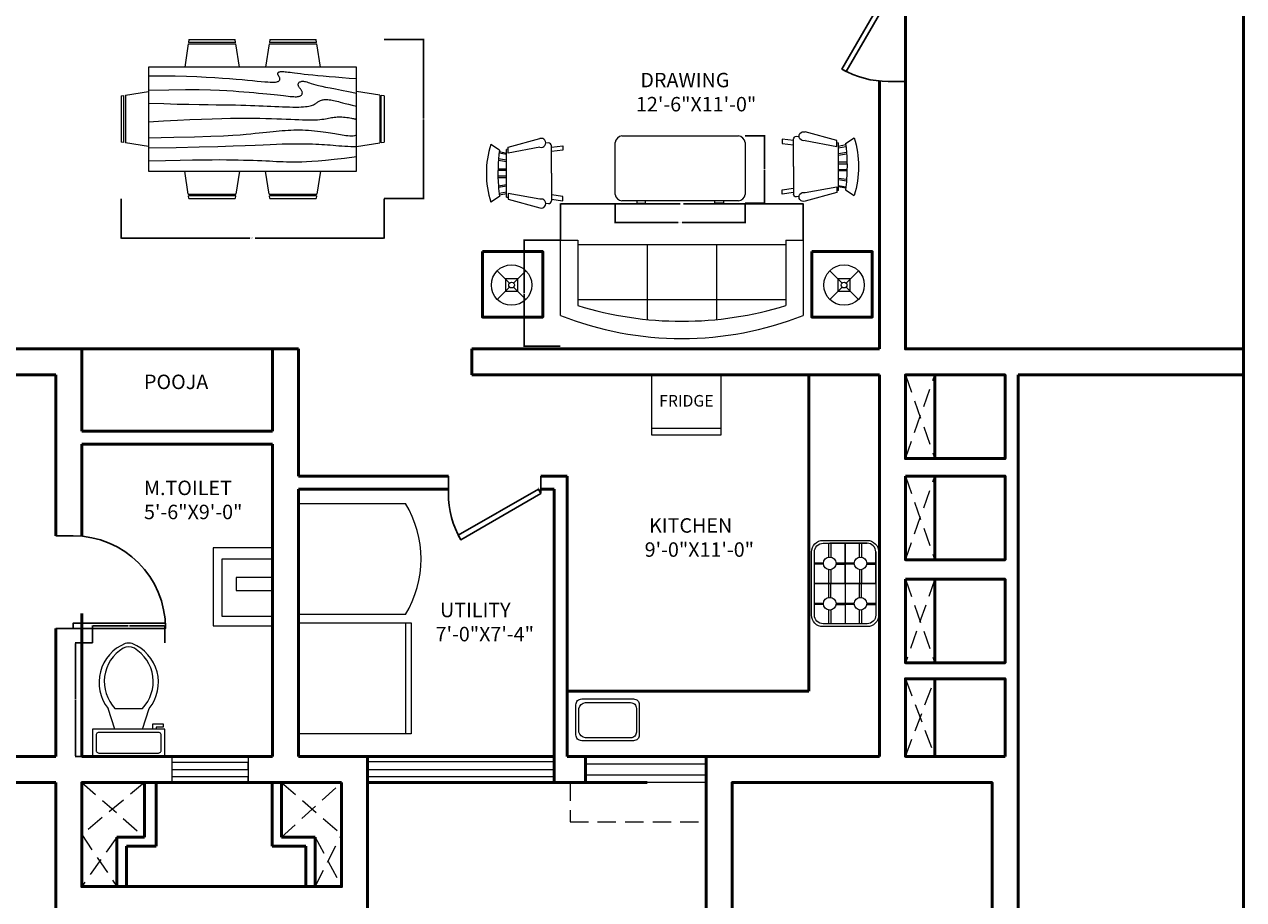
# Model space of a CAD drawing. Units: inches. Extents: x -105 to 1531, y -656 to 2003.
# Tile 4 of 6: x 553 to 975, y 553 to 856. Entities that reach past the tile are written whole.
import ezdxf

# ---------------------------------------------------------------- set-up
doc = ezdxf.new("R2010")
doc.units = ezdxf.units.IN
doc.header["$MEASUREMENT"] = 0
doc.linetypes.add('DASHED', pattern=[19.05, 12.7, -6.35])
for name, color, linetype, lineweight in [('A-ANNO-DIMS', 2, 'Continuous', 18), ('A-AREA-IDEN', 7, 'Continuous', 25), ('A-DOOR', 3, 'Continuous', 25), ('A-FLOR-FIXT', 9, 'Continuous', 18), ('A-FLOR-OVHD', 8, 'DASHED', 18), ('A-FURN', 8, 'Continuous', 18), ('A-GLAZ', 4, 'Continuous', 18), ('A-WALL', 7, 'Continuous', 50)]:
    doc.layers.add(name, color=color, linetype=linetype, lineweight=lineweight)
doc.styles.get("Standard").update_dxf_attribs({"font": 'arial.ttf'})
doc.dimstyles.get("Standard").update_dxf_attribs({"dimtxt": 0.18, "dimasz": 0.18, "dimexe": 0.18, "dimexo": 0.0625, "dimgap": 0.09, "dimtad": 0, "dimtih": 1, "dimtoh": 1, "dimdec": 0, "dimzin": 0, "dimdsep": 46, "dimlunit": 3, "dimtxsty": 'Standard', "dimcen": 0.09, "dimadec": 0, "dimazin": 0, "dimtfac": 1, "dimtdec": 0, "dimtofl": 0, "dimtmove": 0, "dimatfit": 3, "dimfxl": 1, "dimtolj": 1, "dimtzin": 0, "dimarcsym": 0})

# ---------------------------------------------------------------- blocks, each defined once
blk = doc.blocks.new('Dining Set - 36 x 72 in.')
for p, q in [((-22.2343, 26.00059), (-23.4847, 17.99762)), ((-22.2304, 26), (-5.7608, 26)), ((-22, 27.5), (-22.1562, 26.50042)), ((-5.8416, 26.5), (-22.1534, 26.5)), ((-22, 27.5), (-6, 27.5)), ((-5.8437, 26.49966), (-6, 27.5)), ((-4.5152, 17.99762), (-5.7655, 25.99926)), ((5.7657, 26.00059), (4.5153, 17.99762)), ((5.7696, 26), (22.2392, 26)), ((6, 27.5), (5.8438, 26.50042)), ((22.1584, 26.5), (5.8466, 26.5)), ((6, 27.5), (22, 27.5)), ((22.1563, 26.49966), (22, 27.5)), ((23.4848, 17.99762), (22.2345, 25.99926)), ((36, 18), (-36, 18)), ((-36, 18), (-36, -18)), ((36, -18), (36, 18)), ((-44.0006, 8.23428), (-35.9976, 9.48474)), ((44.0006, 8.23428), (35.9976, 9.48474)), ((-45.5, 8), (-44.5004, 8.15617)), ((-45.5, 8), (-45.5, -8)), ((-44.5, -8.15843), (-44.5, 8.15338)), ((-44, 8.23041), (-44, -8.23915)), ((44, 8.23041), (44, -8.23915)), ((44.5, -8.15843), (44.5, 8.15338)), ((45.5, 8), (44.5005, 8.15617)), ((45.5, 8), (45.5, -8)), ((-44.4997, -8.15631), (-45.5, -8)), ((-35.9976, -9.48476), (-43.9993, -8.2345)), ((35.9976, -9.48476), (43.9993, -8.2345)), ((44.4997, -8.15631), (45.5, -8)), ((-36, -18), (36, -18)), ((-22.2343, -26.0006), (-23.4847, -17.99762)), ((-4.5152, -17.99762), (-5.7655, -25.99928)), ((5.7657, -26.0006), (4.5153, -17.99762)), ((23.4848, -17.99762), (22.2345, -25.99928)), ((-22.2304, -26), (-5.7608, -26)), ((-22, -27.5), (-22.1562, -26.50044)), ((-5.8416, -26.5), (-22.1534, -26.5)), ((-22, -27.5), (-6, -27.5)), ((-5.8437, -26.49967), (-6, -27.5)), ((5.7696, -26), (22.2392, -26)), ((6, -27.5), (5.8438, -26.50044)), ((22.1584, -26.5), (5.8466, -26.5)), ((6, -27.5), (22, -27.5)), ((22.1563, -26.49967), (22, -27.5))]:
    blk.add_line(p, q)
for points in [[(-36, 15), (-31.1772, 14.97754), (-26.8079, 14.91406), (-22.8538, 14.81543), (-19.276, 14.6875), (-16.0362, 14.53613), (-13.0957, 14.36718), (-10.4159, 14.18652), (-7.9583, 14), (-5.6904, 13.81315), (-3.6035, 13.63021), (-1.6954, 13.45508), (0.0365, 13.29166), (1.5945, 13.14388), (2.9811, 13.01562), (4.1988, 12.9108), (5.25, 12.83333), (6.1393, 12.78613), (6.8802, 12.76823), (7.4883, 12.77767), (7.9792, 12.8125), (8.3685, 12.87077), (8.6719, 12.95052), (8.9049, 13.0498), (9.0833, 13.16666), (9.2205, 13.29899), (9.3216, 13.44401), (9.3895, 13.59879), (9.4271, 13.76041), (9.4373, 13.92594), (9.4232, 14.09245), (9.3875, 14.257), (9.3333, 14.41666), (9.2638, 14.56917), (9.1836, 14.71484), (9.0975, 14.85465), (9.0104, 14.98958), (8.9272, 15.1206), (8.8529, 15.2487), (8.7922, 15.37483), (8.75, 15.5), (8.7305, 15.62467), (8.7344, 15.74739), (8.7617, 15.86621), (8.8125, 15.97916), (8.8867, 16.08431), (8.9844, 16.17968), (9.1055, 16.26334), (9.25, 16.33333), (9.4189, 16.38802), (9.6172, 16.42708), (9.8506, 16.45052), (10.125, 16.45833), (10.4463, 16.45052), (10.8203, 16.42708), (11.2529, 16.38802), (11.75, 16.33333), (12.3184, 16.26318), (12.9694, 16.17838), (13.7151, 16.07991), (14.5677, 15.96875), (15.5395, 15.84586), (16.6426, 15.71224), (17.8893, 15.56884), (19.2917, 15.41666), (20.859, 15.25667), (22.5879, 15.08984), (24.4721, 14.91715), (26.5052, 14.73958), (28.6809, 14.5581), (30.9929, 14.3737), (33.4347, 14.18733), (36, 14)], [(-36, 10), (-28.9766, 10.14274), (-23.1725, 10.20442), (-18.4241, 10.19775), (-14.5677, 10.13541), (-11.4399, 10.03011), (-8.877, 9.89453), (-6.7154, 9.74137), (-4.7917, 9.58333), (-2.9698, 9.43082), (-1.2246, 9.28515), (0.4415, 9.14534), (2.026, 9.01041), (3.5266, 8.87939), (4.9408, 8.7513), (6.266, 8.62516), (7.5, 8.5), (8.6411, 8.37549), (9.6914, 8.2539), (10.6538, 8.13818), (11.5312, 8.03125), (12.3267, 7.93603), (13.043, 7.85547), (13.6831, 7.79248), (14.25, 7.75), (14.7471, 7.7303), (15.1797, 7.73307), (15.5537, 7.75732), (15.875, 7.80208), (16.1494, 7.86637), (16.3828, 7.94922), (16.5811, 8.04964), (16.75, 8.16666), (16.8944, 8.29915), (17.0143, 8.44531), (17.1089, 8.60319), (17.1771, 8.77083), (17.218, 8.94629), (17.2305, 9.1276), (17.2137, 9.31282), (17.1667, 9.5), (17.0895, 9.6875), (16.987, 9.875), (16.8649, 10.0625), (16.7292, 10.25), (16.5856, 10.4375), (16.4401, 10.625), (16.2985, 10.8125), (16.1667, 11), (16.05, 11.18733), (15.9518, 11.3737), (15.8752, 11.5581), (15.8229, 11.73958), (15.798, 11.91715), (15.8034, 12.08984), (15.842, 12.25667), (15.9167, 12.41666), (16.0295, 12.56836), (16.1784, 12.70833), (16.3605, 12.83268), (16.5729, 12.9375), (16.8127, 13.01888), (17.0768, 13.07291), (17.3625, 13.0957), (17.6667, 13.08333), (17.9894, 13.03312), (18.3418, 12.94726), (18.7382, 12.82918), (19.1927, 12.68229), (19.7195, 12.51001), (20.3327, 12.31575), (21.0465, 12.10294), (21.875, 11.875), (22.8357, 11.63354), (23.959, 11.37304), (25.2786, 11.08618), (26.8282, 10.76562), (28.6414, 10.40405), (30.752, 9.99414), (33.1936, 9.52856), (36, 9)], [(-36, 5.5), (-30.7157, 5.3348), (-26.069, 5.20963), (-21.9946, 5.11767), (-18.4271, 5.05208), (-15.3009, 5.00602), (-12.5508, 4.97265), (-10.1112, 4.94515), (-7.9167, 4.91666), (-5.909, 4.88167), (-4.0586, 4.83984), (-2.3429, 4.79215), (-0.7396, 4.73958), (0.7739, 4.6831), (2.22, 4.6237), (3.6213, 4.56233), (5, 4.5), (6.373, 4.43782), (7.7344, 4.3776), (9.0723, 4.32129), (10.375, 4.27083), (11.6309, 4.22819), (12.8281, 4.19531), (13.9551, 4.17415), (15, 4.16666), (15.954, 4.17448), (16.819, 4.19791), (17.6001, 4.23698), (18.3021, 4.29166), (18.9299, 4.36198), (19.4883, 4.44791), (19.9823, 4.54948), (20.4167, 4.66666), (20.7969, 4.79899), (21.1302, 4.94401), (21.4245, 5.09879), (21.6875, 5.26041), (21.9271, 5.42594), (22.1511, 5.59245), (22.3672, 5.757), (22.5834, 5.91666), (22.8065, 6.06868), (23.0404, 6.21093), (23.2879, 6.34147), (23.5521, 6.45833), (23.8358, 6.55957), (24.142, 6.64323), (24.4735, 6.70735), (24.8334, 6.75), (25.2235, 6.76969), (25.642, 6.76692), (26.0858, 6.74267), (26.5521, 6.69791), (27.0379, 6.63362), (27.5404, 6.55078), (28.0565, 6.45036), (28.5834, 6.33333), (29.1242, 6.19987), (29.7071, 6.04687), (30.3661, 5.87044), (31.1354, 5.66666), (32.0493, 5.43164), (33.142, 5.16146), (34.4475, 4.85221), (36, 4.5)], [(-36, -1), (-30.7915, -0.6591), (-26.0195, -0.38216), (-21.6519, -0.16284), (-17.6563, 0.00521), (-14.0005, 0.12833), (-10.6523, 0.21289), (-7.5796, 0.26522), (-4.75, 0.29166), (-2.134, 0.29793), (0.2878, 0.28711), (2.5317, 0.26163), (4.6146, 0.22396), (6.5529, 0.17651), (8.3633, 0.12174), (10.0623, 0.06209), (11.6667, 0), (13.1899, -0.06201), (14.6341, -0.1211), (15.9982, -0.17432), (17.2813, -0.21875), (18.4823, -0.25147), (19.6003, -0.26953), (20.6343, -0.27002), (21.5834, -0.25), (22.4481, -0.20768), (23.2357, -0.14584), (23.9549, -0.06836), (24.6146, 0.02083), (25.2235, 0.11784), (25.7904, 0.21875), (26.3241, 0.31966), (26.8334, 0.41666), (27.3265, 0.50618), (27.8099, 0.58593), (28.2894, 0.65397), (28.7709, 0.70833), (29.2601, 0.74707), (29.763, 0.76823), (30.2855, 0.76985), (30.8334, 0.75), (31.4088, 0.70784), (31.9994, 0.64713), (32.589, 0.57275), (33.1615, 0.48958), (33.7008, 0.4025), (34.1908, 0.3164), (34.6153, 0.23616), (34.9584, 0.16666), (35.2099, 0.11165), (35.3848, 0.07031), (35.504, 0.04069), (35.5886, 0.02083), (35.6594, 0.00879), (35.7377, 0.0026), (35.8442, 0.00032), (36, 0)], [(-36, -6.5), (-27.1843, -6.31267), (-20.084, -6.1263), (-14.469, -5.9419), (-10.1094, -5.76042), (-6.7752, -5.58285), (-4.2363, -5.41016), (-2.2629, -5.24333), (-0.625, -5.08334), (0.8708, -4.93099), (2.2715, -4.78646), (3.5872, -4.64974), (4.8281, -4.52084), (6.0046, -4.39974), (7.127, -4.28646), (8.2053, -4.18099), (9.25, -4.08334), (10.2705, -3.99382), (11.2734, -3.91407), (12.2647, -3.84603), (13.25, -3.79167), (14.2354, -3.75293), (15.2266, -3.73177), (16.2295, -3.73015), (17.25, -3.75), (18.2912, -3.79248), (19.3451, -3.85547), (20.4009, -3.93604), (21.4479, -4.03125), (22.4754, -4.13819), (23.4727, -4.25391), (24.4289, -4.37549), (25.3334, -4.5), (26.1785, -4.62492), (26.9694, -4.74935), (27.7145, -4.87281), (28.4219, -4.99479), (29.1, -5.11483), (29.7572, -5.23242), (30.4016, -5.34709), (31.0417, -5.45834), (31.6837, -5.56437), (32.3262, -5.65821), (32.9658, -5.73153), (33.599, -5.77604), (34.2224, -5.78345), (34.8327, -5.74545), (35.4264, -5.65373), (36, -5.5)], [(-36, -10), (-26.4022, -9.81299), (-18.4675, -9.62891), (-11.9839, -9.45069), (-6.7396, -9.28125), (-2.5226, -9.12354), (0.8789, -8.98047), (3.6769, -8.85498), (6.0833, -8.75), (8.2767, -8.66765), (10.3021, -8.60677), (12.1712, -8.56543), (13.8958, -8.54167), (15.4876, -8.53353), (16.9583, -8.53907), (18.3197, -8.55632), (19.5834, -8.58334), (20.7616, -8.61841), (21.8685, -8.66081), (22.9188, -8.71004), (23.9271, -8.76563), (24.9081, -8.82707), (25.8763, -8.89388), (26.8465, -8.96558), (27.8334, -9.04167), (28.8474, -9.12118), (29.8828, -9.20117), (30.93, -9.27824), (31.9792, -9.34896), (33.0205, -9.40991), (34.0443, -9.45768), (35.0407, -9.48885), (36, -9.5)], [(-36, -14.5), (-30.0881, -14.33513), (-25.0332, -14.21224), (-20.7312, -14.12647), (-17.0781, -14.07292), (-13.97, -14.04671), (-11.3027, -14.04297), (-8.9724, -14.05681), (-6.875, -14.08334), (-4.9224, -14.11833), (-3.0905, -14.16016), (-1.3709, -14.20785), (0.2448, -14.26042), (1.7647, -14.3169), (3.1973, -14.3763), (4.5507, -14.43767), (5.8333, -14.5), (7.0554, -14.5621), (8.235, -14.62175), (9.3922, -14.67652), (10.5469, -14.72396), (11.7192, -14.76164), (12.929, -14.78711), (14.1965, -14.79794), (15.5417, -14.79167), (16.9933, -14.76424), (18.6152, -14.70508), (20.4804, -14.60197), (22.6615, -14.44271), (25.2312, -14.21509), (28.2624, -13.9069), (31.8277, -13.50594), (36, -13)]]:
    blk.add_lwpolyline(points)
blk = doc.blocks.new('Sofa - Roundback 7 ft.')
for p, q in [((-12.00002, -32.4421), (-12.00003, -6.5971)), ((11.99997, -32.4421), (11.99998, -6.5971)), ((-36.000027, -34), (-36.000027, -11.4696)), ((35.99998, -34), (35.99998, -11.4696)), ((-35.999844, -13.3819), (35.9998, -13.3819)), ((-36.000027, -32.4421), (35.99998, -32.4421))]:
    blk.add_line(p, q)
for points in [[(-36.000027, -34), (-42.000027, -34), (-42.000027, -8)], [(41.99998, -8), (41.99998, -34), (35.99998, -34)]]:
    blk.add_lwpolyline(points)
for centre, radius, start, end in [((0, -114.25), 114.25, 68.43141, 111.5686), ((-0.00001, -127.1968), 121.1968, 72.72033, 107.2797)]:
    blk.add_arc(centre, radius, start, end)
blk = doc.blocks.new('Chair - Rocking')
for p, q in [((-8, -4.5), (-10, -1.5)), ((-4.5, -7), (-4.96674, -4.19951)), ((-4, -7), (-4.40532, -4.16272)), ((-1.5, -4.05012), (-1.5, -7)), ((-1, -7), (-1, -4.05012)), ((1, -7), (1, -4.04655)), ((1.5, -4.05012), (1.5, -7)), ((4, -7), (4.40187, -4.18694)), ((4.5, -7), (4.96761, -4.19437)), ((8, -4.5), (10, -1.5)), ((-9, -7.5), (-12, -18.49999)), ((-7, -7.5), (-9, -7.5)), ((-9, -18.49999), (-7, -7.5)), ((-8.23428, -6.99939), (-8.3093, -7.47958)), ((-8.23041, -7), (8.23915, -7)), ((-7.5, -4.5), (-7, -7)), ((-6.5, -7), (-7.02225, -4.43)), ((6.5, -7), (7, -4.4057)), ((7.5, -4.5), (7, -7)), ((7, -7.5), (9, -7.5)), ((9, -18.49999), (7, -7.5)), ((8.31071, -7.48854), (8.23449, -7.00073)), ((9, -7.5), (12, -18.49999)), ((-10.36644, -20.64523), (-10.5, -21.49999)), ((10.5, -21.49999), (10.3575, -20.58798)), ((-9, -22.49999), (-9.5, -26.49999)), ((0, -22.49999), (-9.5, -22.49999)), ((-8, -26.49999), (-7.5, -22.49999)), ((0, -22.49999), (9.5, -22.49999)), ((8, -26.49999), (7.5, -22.49999)), ((9, -22.49999), (9.5, -26.49999)), ((-9.5, -26.49999), (-8, -26.49999)), ((9.5, -26.49999), (8, -26.49999))]:
    blk.add_line(p, q)
for centre, radius, start, end in [((0, -34.08333), 34.08333, 72.93847, 107.0615), ((0, -68.25004), 64.25, 93.92211, 97.15267), ((0, -68.25004), 64.25, 82.84733, 93.92211), ((-10.5, -18.99999), 1.58114, 161.5651, 18.43495), ((10.5, -18.99999), 1.58114, 161.5651, 18.43495), ((-9.5, -21.49999), 1, 180, 270), ((9.5, -21.49999), 1, 270, 0)]:
    blk.add_arc(centre, radius, start, end)
blk = doc.blocks.new('Desk - 30 x 60 in.')
for p, q in [((-26.999995, 0), (26.999995, 0)), ((-29.999995, -27), (-29.999995, -3)), ((29.999995, -3), (29.999995, -27)), ((26.999995, -30), (-26.999995, -30)), ((-20.000005, -30), (-20.000005, -31)), ((-20.000005, -31), (-16.000005, -31)), ((-16.000005, -31), (-16.000005, -30)), ((15.999995, -31), (15.999995, -30)), ((19.999995, -31), (15.999995, -31)), ((19.999995, -30), (19.999995, -31))]:
    blk.add_line(p, q)
for centre, start, end in [((-26.499995, -3.5), 98.1301, 171.8699), ((26.499995, -3.5), 8.130102, 81.8699), ((-26.499995, -26.5), 188.1301, 261.8699), ((26.499995, -26.5), 278.1301, 351.8699)]:
    blk.add_arc(centre, 3.535534, start, end)
blk = doc.blocks.new('Lamp - Table')
for p, q in [((0, 7), (0, 1)), ((-1, 0), (-7, 0)), ((0, 3), (-3, 0)), ((-3, 0), (0, -3)), ((3, 0), (0, 3)), ((0, -3), (3, 0)), ((1, 0), (7, 0)), ((0, -1), (0, -7))]:
    blk.add_line(p, q)
for radius in [7, 1]:
    blk.add_circle((0, 0), radius)
blk = doc.blocks.new('*U11')
for p, q in [((0, 0), (0, 6)), ((32, 0), (32, 6))]:
    blk.add_line(p, q)
blk.add_lwpolyline([(0, 0), (27.71, -16), (28.59, -14.48), (0.88, 1.52)], close=True)
blk.add_arc((0, 0), 32, 330, 0)
blk = doc.blocks.new('Toilet - top')
for p, q in [((9.5, -6), (9.5, -2)), ((-10, -8.5), (-8, -8.5)), ((-10, -9.5), (-10, -8.5)), ((-7, -9.5), (-10, -9.5)), ((-8, -8.5), (-8, -8)), ((-7, -8), (-7, -9.5)), ((-4, -8), (-6, -14)), ((4, -8), (6, -14)), ((4, -14), (-4, -14))]:
    blk.add_line(p, q)
blk.add_lwpolyline([(10.5, -8), (10.5, 0), (-10.5, 0), (-10.5, -8)], close=True)
for points in [[(-9.5, -2), (-9.5, -6)], [(8.5, -1), (-8.5, -1)], [(-8.5, -7), (8.5, -7)]]:
    blk.add_lwpolyline(points)
for centre, radius, start, end in [((-8.62, -1.88), 0.884, 81.8699, 188.1301), ((8.62, -1.88), 0.884, 351.8699, 98.1301), ((-8.62, -6.12), 0.884, 171.8699, 278.1301), ((8.62, -6.12), 0.884, 261.8699, 8.1301), ((3.52, -21.58), 12.17, 141.4691, 247.9714), ((4.2, -21.82), 11.33, 136.3677, 238.9468), ((-3.52, -21.58), 12.17, 292.0284, 38.5307), ((-4.2, -21.82), 11.33, 301.053, 43.6321), ((0, -27.88), 4, 245.7318, 294.2682), ((0, -29), 4, 254.8605, 285.1395)]:
    blk.add_arc(centre, radius, start, end)
blk = doc.blocks.new('*U12')
for p, q in [((-32, 0), (-32, -6)), ((0, 0), (0, -6))]:
    blk.add_line(p, q)
blk.add_lwpolyline([(0, 0), (0, 32), (-1.75, 32), (-1.75, 0)], close=True)
blk.add_arc((0, 0), 32, 90, 180)
blk = doc.blocks.new('*U2')
for p, q in [((-32, 0), (-32, 6)), ((0, 0), (0, 6))]:
    blk.add_line(p, q)
blk.add_lwpolyline([(0, 0), (-27.71, -16), (-28.59, -14.48), (-0.88, 1.52)], close=True)
blk.add_arc((0, 0), 32, 180, 210)
blk = doc.blocks.new('*D25')
at = {"layer": 'A-ANNO-DIMS', "color": 0, "lineweight": -2, "transparency": 16777216}
for p, q in [((738.64, 781.2), (738.64, 793.91)), ((738.82, 793.73), (780.04, 793.73)), ((822.46, 793.73), (781.23, 793.73)), ((822.64, 781.2), (822.64, 793.91))]:
    blk.add_line(p, q, dxfattribs=at)
at = {"layer": 'A-ANNO-DIMS', "color": 0, "transparency": 16777216}
for points in [[(738.82, 793.76), (738.82, 793.7), (738.64, 793.73)], [(822.46, 793.76), (822.46, 793.7), (822.64, 793.73)]]:
    blk.add_solid(points, dxfattribs=at)
at = {"layer": 'Defpoints', "color": 0, "transparency": 16777216}
for p in [(738.64, 793.73), (738.64, 781.13), (822.64, 781.13)]:
    blk.add_point(p, dxfattribs=at)
at = {"layer": 'A-ANNO-DIMS', "color": 0, "transparency": 16777216, "insert": (780.64, 793.73), "char_height": 0.18, "attachment_point": 5}
blk.add_mtext('\\A1;SOFA 84', dxfattribs=at)
blk = doc.blocks.new('*D26')
at = {"layer": 'A-ANNO-DIMS', "color": 0, "lineweight": -2, "transparency": 16777216}
for p, q in [((738.57, 781.13), (725.86, 781.13)), ((726.04, 780.95), (726.04, 762.98)), ((726.04, 744.65), (726.04, 762.62)), ((738.57, 744.47), (725.86, 744.47))]:
    blk.add_line(p, q, dxfattribs=at)
at = {"layer": 'A-ANNO-DIMS', "color": 0, "transparency": 16777216}
for points in [[(726.01, 780.95), (726.07, 780.95), (726.04, 781.13)], [(726.01, 744.65), (726.07, 744.65), (726.04, 744.47)]]:
    blk.add_solid(points, dxfattribs=at)
at = {"layer": 'Defpoints', "color": 0, "transparency": 16777216}
for p in [(738.64, 781.13), (726.04, 744.47), (738.64, 744.47)]:
    blk.add_point(p, dxfattribs=at)
at = {"layer": 'A-ANNO-DIMS', "color": 0, "transparency": 16777216, "insert": (726.04, 762.8), "char_height": 0.18, "attachment_point": 5}
blk.add_mtext('\\A1;37', dxfattribs=at)
blk = doc.blocks.new('*D29')
at = {"layer": 'A-ANNO-DIMS', "color": 0, "lineweight": -2, "transparency": 16777216}
for p, q in [((576.72, 641.83), (570.71, 641.83)), ((570.89, 641.65), (570.89, 622.38)), ((570.89, 602.75), (570.89, 622.02)), ((576.72, 602.57), (570.71, 602.57))]:
    blk.add_line(p, q, dxfattribs=at)
at = {"layer": 'A-ANNO-DIMS', "color": 0, "transparency": 16777216}
for points in [[(570.86, 641.65), (570.92, 641.65), (570.89, 641.83)], [(570.86, 602.75), (570.92, 602.75), (570.89, 602.57)]]:
    blk.add_solid(points, dxfattribs=at)
at = {"layer": 'Defpoints', "color": 0, "transparency": 16777216}
for p in [(576.78, 641.83), (570.89, 602.57), (576.78, 602.57)]:
    blk.add_point(p, dxfattribs=at)
at = {"layer": 'A-ANNO-DIMS', "color": 0, "transparency": 16777216, "insert": (570.89, 622.2), "char_height": 0.18, "attachment_point": 5}
blk.add_mtext('\\A1;WC 39', dxfattribs=at)
blk = doc.blocks.new('*D30')
at = {"layer": 'A-ANNO-DIMS', "color": 0, "lineweight": -2, "transparency": 16777216}
for p, q in [((576.78, 641.89), (576.78, 647.9)), ((576.96, 647.72), (589.04, 647.72)), ((601.55, 647.72), (589.48, 647.72)), ((601.73, 641.89), (601.73, 647.9))]:
    blk.add_line(p, q, dxfattribs=at)
at = {"layer": 'A-ANNO-DIMS', "color": 0, "transparency": 16777216}
for points in [[(576.96, 647.75), (576.96, 647.69), (576.78, 647.72)], [(601.55, 647.75), (601.55, 647.69), (601.73, 647.72)]]:
    blk.add_solid(points, dxfattribs=at)
at = {"layer": 'Defpoints', "color": 0, "transparency": 16777216}
for p in [(576.78, 647.72), (576.78, 641.83), (601.73, 641.83)]:
    blk.add_point(p, dxfattribs=at)
at = {"layer": 'A-ANNO-DIMS', "color": 0, "transparency": 16777216, "insert": (589.26, 647.72), "char_height": 0.18, "attachment_point": 5}
blk.add_mtext('\\A1;25', dxfattribs=at)
blk = doc.blocks.new('*D35')
at = {"layer": 'A-ANNO-DIMS', "color": 0, "lineweight": -2, "transparency": 16777216}
for p, q in [((757.58, 793.96), (757.58, 787.1)), ((802.51, 793.96), (802.51, 787.1)), ((757.76, 787.28), (779.39, 787.28)), ((802.33, 787.28), (780.7, 787.28))]:
    blk.add_line(p, q, dxfattribs=at)
at = {"layer": 'A-ANNO-DIMS', "color": 0, "transparency": 16777216}
for points in [[(757.76, 787.31), (757.76, 787.25), (757.58, 787.28)], [(802.33, 787.31), (802.33, 787.25), (802.51, 787.28)]]:
    blk.add_solid(points, dxfattribs=at)
at = {"layer": 'Defpoints', "color": 0, "transparency": 16777216}
for p in [(757.58, 794.02), (802.51, 794.02), (802.51, 787.28)]:
    blk.add_point(p, dxfattribs=at)
at = {"layer": 'A-ANNO-DIMS', "color": 0, "transparency": 16777216, "insert": (780.05, 787.28), "char_height": 0.18, "attachment_point": 5}
blk.add_mtext('\\A1;TABLE 45', dxfattribs=at)
blk = doc.blocks.new('*D36')
at = {"layer": 'A-ANNO-DIMS', "color": 0, "lineweight": -2, "transparency": 16777216}
for p, q in [((802.58, 817.24), (809.43, 817.24)), ((809.25, 817.06), (809.25, 805.81)), ((809.25, 794.2), (809.25, 805.45)), ((802.58, 794.02), (809.43, 794.02))]:
    blk.add_line(p, q, dxfattribs=at)
at = {"layer": 'A-ANNO-DIMS', "color": 0, "transparency": 16777216}
for points in [[(809.22, 817.06), (809.28, 817.06), (809.25, 817.24)], [(809.22, 794.2), (809.28, 794.2), (809.25, 794.02)]]:
    blk.add_solid(points, dxfattribs=at)
at = {"layer": 'Defpoints', "color": 0, "transparency": 16777216}
for p in [(802.51, 817.24), (809.25, 817.24), (802.51, 794.02)]:
    blk.add_point(p, dxfattribs=at)
at = {"layer": 'A-ANNO-DIMS', "color": 0, "transparency": 16777216, "insert": (809.25, 805.63), "char_height": 0.18, "attachment_point": 5}
blk.add_mtext('\\A1;23', dxfattribs=at)
blk = doc.blocks.new('*D39')
at = {"layer": 'A-ANNO-DIMS', "color": 0, "lineweight": -2, "transparency": 16777216}
for p, q in [((586.61, 795.5), (586.61, 781.73)), ((677.61, 795.5), (677.61, 781.73)), ((586.79, 781.91), (631.16, 781.91)), ((677.43, 781.91), (633.06, 781.91))]:
    blk.add_line(p, q, dxfattribs=at)
at = {"layer": 'A-ANNO-DIMS', "color": 0, "transparency": 16777216}
for points in [[(586.79, 781.94), (586.79, 781.88), (586.61, 781.91)], [(677.43, 781.94), (677.43, 781.88), (677.61, 781.91)]]:
    blk.add_solid(points, dxfattribs=at)
at = {"layer": 'Defpoints', "color": 0, "transparency": 16777216}
for p in [(586.61, 795.56), (677.61, 795.56), (677.61, 781.91)]:
    blk.add_point(p, dxfattribs=at)
at = {"layer": 'A-ANNO-DIMS', "color": 0, "transparency": 16777216, "insert": (632.11, 781.91), "char_height": 0.18, "attachment_point": 5}
blk.add_mtext('\\A1;DINING SET 91', dxfattribs=at)
blk = doc.blocks.new('*D40')
at = {"layer": 'A-ANNO-DIMS', "color": 0, "lineweight": -2, "transparency": 16777216}
for p, q in [((677.67, 850.56), (691.44, 850.56)), ((691.26, 850.38), (691.26, 823.24)), ((691.26, 795.74), (691.26, 822.88)), ((677.67, 795.56), (691.44, 795.56))]:
    blk.add_line(p, q, dxfattribs=at)
at = {"layer": 'A-ANNO-DIMS', "color": 0, "transparency": 16777216}
for points in [[(691.23, 850.38), (691.29, 850.38), (691.26, 850.56)], [(691.23, 795.74), (691.29, 795.74), (691.26, 795.56)]]:
    blk.add_solid(points, dxfattribs=at)
at = {"layer": 'Defpoints', "color": 0, "transparency": 16777216}
for p in [(677.61, 850.56), (691.26, 850.56), (677.61, 795.56)]:
    blk.add_point(p, dxfattribs=at)
at = {"layer": 'A-ANNO-DIMS', "color": 0, "transparency": 16777216, "insert": (691.26, 823.06), "char_height": 0.18, "attachment_point": 5}
blk.add_mtext('\\A1;55', dxfattribs=at)

msp = doc.modelspace()

# ---------------------------------------------------------------- linework, layer by layer
at = {"layer": 'A-FLOR-FIXT'}
for p, q in [((831.46, 671.51), (831.46, 676.31)), ((832.17, 676.31), (832.17, 671.5)), ((842.09, 671.51), (842.09, 676.31)), ((842.8, 676.31), (842.8, 671.5)), ((832.17, 667.21), (832.17, 662.4)), ((833.98, 669.57), (837.12, 669.57)), ((833.98, 669.15), (837.12, 669.15)), ((842.8, 667.21), (842.8, 662.4)), ((844.61, 669.57), (847.75, 669.57)), ((844.61, 669.15), (847.75, 669.15)), ((831.46, 662.56), (831.46, 662.27)), ((831.46, 657.55), (831.46, 662.36)), ((842.09, 662.56), (842.09, 662.27)), ((842.09, 657.55), (842.09, 662.36)), ((833.98, 655.61), (837.12, 655.61)), ((833.98, 655.2), (837.12, 655.2)), ((844.61, 655.61), (847.75, 655.61)), ((844.61, 655.2), (847.75, 655.2)), ((831.46, 648.48), (831.46, 653.25)), ((832.17, 653.25), (832.17, 648.48)), ((842.09, 648.48), (842.09, 653.25)), ((842.8, 653.25), (842.8, 648.48))]:
    msp.add_line(p, q, dxfattribs=at)
for points in [[(844.75, 677.31, -0.414214), (848.75, 673.31), (848.75, 651.48, -0.414214), (844.75, 647.48), (829.49, 647.48, -0.414214), (825.49, 651.48), (825.49, 673.31, -0.414214), (829.49, 677.31), (837.12, 677.31)], [(745.98, 622.49), (763.92, 622.49, -0.414214), (765.92, 620.49), (765.92, 610.02, -0.414214), (763.92, 608.02), (745.98, 608.02, -0.414214), (743.98, 610.02), (743.98, 620.49, -0.414214)], [(747.3, 621.2), (762.91, 621.2, -0.414214), (764.91, 619.2), (764.91, 611.03, -0.414214), (762.91, 609.03), (747.3, 609.03, -0.307149), (744.95, 611.03), (744.95, 619.2, -0.307149)]]:
    msp.add_lwpolyline(points, format="xyb", close=True, dxfattribs=at)
for points in [[(842.09, 667.2), (842.09, 662.4), (842.44, 662.4), (837.12, 662.4), (847.75, 662.4), (847.75, 673.31), (847.75, 651.48, -0.414214), (844.75, 648.48), (829.49, 648.48, -0.414214), (826.49, 651.48), (826.49, 673.31, -0.414214), (829.49, 676.31), (837.12, 676.31), (837.12, 648.48)], [(847.75, 669.36), (847.75, 673.31, 0.414214), (844.75, 676.31), (842.44, 676.31)]]:
    msp.add_lwpolyline(points, format="xyb", dxfattribs=at)
for points in [[(826.49, 662.4), (837.12, 662.4), (837.12, 676.31), (831.81, 676.31)], [(829.49, 676.31), (844.75, 676.31), (837.12, 676.31), (837.12, 669.36)], [(829.64, 669.15), (826.49, 669.15), (826.49, 669.36), (826.49, 669.57), (829.64, 669.57)], [(847.75, 662.4), (826.49, 662.4), (831.81, 662.4), (831.46, 662.4), (831.46, 667.2)], [(840.27, 669.15), (837.12, 669.15), (837.12, 669.36), (837.12, 669.57), (840.27, 669.57)], [(832.17, 657.55), (832.17, 662.36), (832.17, 662.49)], [(842.8, 657.55), (842.8, 662.36), (842.8, 662.49)], [(829.64, 655.2), (826.49, 655.2), (826.49, 655.4), (826.49, 655.61), (829.64, 655.61)], [(840.27, 655.2), (837.12, 655.2), (837.12, 655.4), (837.12, 655.61), (840.27, 655.61)]]:
    msp.add_lwpolyline(points, dxfattribs=at)
for points in [[(639, 674.76), (618.53, 674.76), (618.53, 647.74), (639, 647.74)], [(639, 670.85), (621.49, 670.85), (621.49, 651.08), (639, 651.08)], [(639, 664.48), (626.4, 664.48), (626.4, 660.01), (639, 660.01)]]:
    msp.add_lwpolyline(points, close=True, dxfattribs=at)
for centre in [(831.81, 669.36), (842.44, 669.36), (831.81, 655.4), (842.44, 655.4)]:
    msp.add_circle(centre, 2.18, dxfattribs=at)
at = {"layer": 'A-FLOR-OVHD', "ltscale": 0.5}
for p, q in [((858, 734.57), (868.16, 705.64)), ((858, 705.64), (868.16, 734.57)), ((858, 699.57), (868.16, 670.64)), ((858, 670.64), (868.16, 699.57)), ((858, 663.89), (868.16, 634.97)), ((868.16, 663.89), (858, 634.97)), ((858, 629.44), (868.16, 602.57)), ((858, 602.57), (868.16, 629.44)), ((573, 593.57), (594.75, 574.68)), ((594.75, 593.57), (573, 575.57)), ((642.13, 593.57), (662.93, 575.57)), ((642.13, 574.68), (662.93, 593.57)), ((741.97, 593.57), (741.97, 580.01)), ((741.97, 580.01), (789, 580.01)), ((573, 575.57), (585.14, 557.57)), ((585.14, 574.68), (573, 557.57)), ((653.72, 557.57), (662.93, 575.57)), ((653.72, 574.68), (662.93, 557.57))]:
    msp.add_line(p, q, dxfattribs=at)
at = {"layer": 'A-FURN'}
for p, q in [((770.29, 716.15), (794.11, 716.15)), ((682.59, 648.82), (684.99, 648.82)), ((684.99, 648.82), (684.99, 610.39))]:
    msp.add_line(p, q, dxfattribs=at)
for points in [[(770.29, 734.57), (794.11, 734.57), (794.11, 713.75), (770.29, 713.75)], [(648, 648.82), (686.98, 648.82), (686.98, 610.39), (648, 610.39)]]:
    msp.add_lwpolyline(points, close=True, dxfattribs=at)
msp.add_lwpolyline([(684.99, 651.68), (648, 651.68), (648, 690.11), (684.99, 690.11)], dxfattribs=at)
msp.add_arc((653.67, 670.89), 36.74, 328.4696, 31.5304, dxfattribs=at)
at = {"layer": 'A-GLAZ'}
for p, q in [((604.32, 593.57), (604.32, 602.57)), ((604.32, 602.57), (630.64, 602.57)), ((630.64, 600.49), (604.32, 600.49)), ((630.64, 602.57), (630.64, 593.57)), ((630.64, 598.07), (630.64, 600.49)), ((736.5, 600.72), (671.93, 600.72)), ((747.33, 598.07), (747.33, 600.07)), ((747.33, 600.07), (789, 600.07)), ((604.32, 595.55), (604.32, 598.07)), ((604.32, 598.07), (630.64, 598.07)), ((630.64, 595.55), (604.32, 595.55)), ((630.64, 593.57), (630.64, 595.55)), ((671.93, 598.07), (736.5, 598.07)), ((736.5, 595.52), (671.93, 595.52)), ((747.33, 596.27), (789, 596.27)), ((789, 593.57), (768.63, 593.57))]:
    msp.add_line(p, q, dxfattribs=at)
at = {"layer": 'A-WALL'}
for p, q in [((858, 743.57), (858, 1039.57)), ((975, 743.57), (975, 919.57)), ((975, 625.97), (975, 919.57)), ((849, 743.57), (849, 836.21)), ((648, 743.57), (509, 743.57)), ((573, 715.07), (573, 743.57)), ((639, 715.07), (639, 743.57)), ((648, 699.57), (648, 743.57)), ((708, 743.57), (708, 734.57)), ((849, 743.57), (708, 743.57)), ((860, 743.57), (858, 743.57)), ((860, 743.57), (897, 743.57)), ((975, 743.57), (975, 220.07)), ((564, 734.57), (392, 734.57)), ((564, 678.9), (564, 734.57)), ((849, 734.57), (708, 734.57)), ((824.57, 734.57), (824.57, 643.1)), ((849, 602.57), (849, 734.57)), ((849, 602.57), (849, 734.57)), ((858, 734.57), (892.5, 734.57)), ((860, 734.57), (858, 734.57)), ((858, 705.64), (858, 734.57)), ((865.59, 734.57), (865.59, 734.57)), ((865.59, 734.57), (868.16, 734.57)), ((868.16, 734.57), (868.16, 705.64)), ((892.5, 705.64), (892.5, 734.57)), ((897, 734.57), (897, 602.57)), ((639, 715.07), (573, 715.07)), ((639, 710.57), (573, 710.57)), ((573, 678.76), (573, 710.57)), ((639, 602.57), (639, 710.57)), ((699.87, 699.57), (648, 699.57)), ((741, 699.57), (731.87, 699.57)), ((741, 602.57), (741, 699.57)), ((860, 699.57), (858, 699.57)), ((858, 670.64), (858, 699.57)), ((868.16, 699.57), (868.16, 670.64)), ((892.5, 670.64), (892.5, 699.57)), ((648, 602.57), (648, 695.07)), ((699.87, 695.07), (648, 695.07)), ((731, 695.07), (730.97, 695.07)), ((736.5, 695.07), (731.87, 695.07)), ((736.5, 602.57), (736.5, 695.07)), ((858, 634.97), (858, 663.89)), ((868.16, 663.89), (868.16, 634.97)), ((892.5, 634.97), (892.5, 663.89)), ((573, 602.57), (573, 652.09)), ((564, 602.57), (564, 646.9)), ((824.57, 643.1), (824.57, 625.17)), ((858, 602.57), (858, 629.44)), ((868.16, 629.44), (868.16, 602.57)), ((892.5, 602.57), (892.5, 629.44)), ((824.57, 625.17), (741, 625.17)), ((564, 602.57), (392, 602.57)), ((639, 602.57), (573, 602.57)), ((736.5, 602.57), (648, 602.57)), ((671.93, 593.57), (671.93, 602.57)), ((736.5, 602.57), (736.5, 593.57)), ((736.5, 598.07), (736.5, 600.72)), ((741.83, 602.57), (741, 602.57)), ((773.83, 602.57), (741.83, 602.57)), ((747.33, 602.57), (747.33, 593.57)), ((849, 602.57), (773.83, 602.57)), ((892.5, 602.57), (858, 602.57)), ((860, 602.57), (858, 602.57)), ((861, 602.57), (860, 602.57)), ((892.5, 602.57), (861, 602.57)), ((671.93, 595.52), (671.93, 598.07)), ((736.5, 593.57), (736.5, 595.52)), ((564, 593.57), (383, 593.57)), ((573, 593.57), (573, 557.57)), ((662.93, 593.57), (573, 593.57)), ((594.75, 574.68), (594.75, 593.57)), ((594.75, 593.57), (598.8, 593.57)), ((598.8, 593.57), (598.8, 571.52)), ((638.84, 593.57), (638.84, 571.52)), ((642.13, 574.68), (642.13, 593.57)), ((741.97, 593.57), (671.93, 593.57)), ((768.63, 593.57), (741.97, 593.57)), ((888, 593.57), (798, 593.57)), ((585.14, 571.77), (585.14, 574.68)), ((585.14, 574.68), (594.75, 574.68)), ((643.48, 574.68), (642.13, 574.68)), ((642.13, 574.68), (653.72, 574.68)), ((653.72, 574.68), (653.72, 557.57)), ((585.14, 557.57), (585.14, 571.77)), ((598.8, 571.52), (588.5, 571.52)), ((588.5, 571.52), (588.5, 557.57)), ((638.84, 571.52), (650.55, 571.52)), ((650.55, 571.52), (650.55, 557.57)), ((647.42, 557.57), (651.35, 557.57))]:
    msp.add_line(p, q, dxfattribs=at)
for points in [[(975, 919.57), (858, 919.57), (858, 743.57), (975, 743.57)], [(849, 836.21), (849, 743.57)], [(858, 705.64), (858, 734.57), (892.5, 734.57)], [(858, 734.57), (892.5, 734.57)], [(897, 734.57), (897, 602.57)], [(897, 734.57), (975, 734.57)], [(858, 670.64), (858, 699.57)], [(858, 634.97), (858, 663.89)], [(892.5, 602.57), (858, 602.57), (858, 629.44)], [(858, 602.57), (858, 629.44), (892.5, 629.44), (892.5, 602.57)], [(639, 602.57), (573, 602.57)], [(671.93, 602.57), (648, 602.57)], [(888, 464.57), (789, 464.57), (789, 602.57), (849, 602.57)], [(858, 602.57), (892.5, 602.57)], [(897, 602.57), (897, 464.57)], [(564, 593.57), (564, 548.57), (671.93, 548.57), (671.93, 593.57)], [(576.45, 557.57), (587.25, 557.57)], [(597.91, 557.57), (608.72, 557.57)], [(608.72, 557.57), (619.52, 557.57)], [(619.52, 557.57), (630.32, 557.57)], [(630.32, 557.57), (641.12, 557.57)], [(641.12, 557.57), (651.92, 557.57)]]:
    msp.add_lwpolyline(points, dxfattribs=at)
for points in [[(711.61, 777.23), (732.5, 777.23), (732.5, 754.57), (711.61, 754.57)], [(825.61, 777.23), (846.5, 777.23), (846.5, 754.57), (825.61, 754.57)], [(858, 734.57), (892.5, 734.57), (892.5, 705.64), (858, 705.64)], [(858, 699.57), (892.5, 699.57), (892.5, 670.64), (858, 670.64)], [(858, 663.89), (892.5, 663.89), (892.5, 634.97), (858, 634.97)], [(662.93, 593.57), (573, 593.57), (573, 557.57), (662.93, 557.57)], [(888, 473.57), (798, 473.57), (798, 593.57), (888, 593.57)]]:
    msp.add_lwpolyline(points, close=True, dxfattribs=at)

# ---------------------------------------------------------------- block references
at = {"layer": 'A-DOOR', "rotation": 270}
for name, p in [('*U11', (852, 868.07)), ('*U12', (570, 646.9))]:
    msp.add_blockref(name, p, dxfattribs=at)
at = {"layer": 'A-DOOR'}
msp.add_blockref('*U2', (731.87, 693.57), dxfattribs=at)
at = {"layer": 'A-FLOR-FIXT', "xscale": 1.188190600298337, "yscale": 1.188190600298337, "zscale": 1.188190600298337, "rotation": 180}
msp.add_blockref('Toilet - top', (589.26, 602.57), dxfattribs=at)
at = {"layer": 'A-FURN'}
msp.add_blockref('Dining Set - 36 x 72 in.', (632.11, 823.06), dxfattribs=at)
at = {"layer": 'A-FURN', "xscale": -1, "rotation": 270.0000177856219}
msp.add_blockref('Chair - Rocking', (841.79, 806.62), dxfattribs=at)
at = {"layer": 'A-FURN'}
for name, p, rotation in [('Chair - Rocking', (713.01, 804.31), 89.99998221437814), ('Sofa - Roundback 7 ft.', (780.64, 747.13), 180), ('Lamp - Table', (721.73, 765.64), 315.0000286478754), ('Lamp - Table', (836.76, 765.64), 315.0000286478754)]:
    msp.add_blockref(name, p, dxfattribs=dict(at, rotation=rotation))
at = {"layer": 'A-FURN', "xscale": 0.7489552448081258, "yscale": 0.7489552448081258, "zscale": 0.7489552448081258}
msp.add_blockref('Desk - 30 x 60 in.', (780.05, 817.24), dxfattribs=at)

# ---------------------------------------------------------------- texts
at = {"layer": 'A-AREA-IDEN', "ltscale": 5, "attachment_point": 1}
for s, insert, char_height in [(' DRAWING\\P12\'-6"X11\'-0"', (764.77, 839.05), 5), ('POOJA', (594.55, 734.66), 5), ('FRIDGE', (772.81, 727.61), 4), ('M.TOILET\\P5\'-6"X9\'-0"', (594.55, 697.99), 5), (' KITCHEN\\P9\'-0"X11\'-0"', (767.78, 684.98), 5), (' UTILITY\\P7\'-0"X7\'-4"', (695.44, 655.75), 5)]:
    msp.add_mtext_dynamic_manual_height_columns(s, width=114.6643, gutter_width=1, heights=[0], dxfattribs=dict(at, insert=insert, char_height=char_height))

# ---------------------------------------------------------------- dimensions: what is measured, and where the dimension line sits
at = {"layer": 'A-ANNO-DIMS'}
for base, p1, p2, angle, picture, middle in [((691.26, 850.56), (677.61, 795.56), (677.61, 850.56), 90, '*D40', (691.26, 823.06)), ((809.25, 817.24), (802.51, 794.02), (802.51, 817.24), 90, '*D36', (809.25, 805.63)), ((726.04, 744.47), (738.64, 781.13), (738.64, 744.47), 270, '*D26', (726.04, 762.8)), ((576.78, 647.72), (601.73, 641.83), (576.78, 641.83), 180, '*D30', (589.26, 647.72))]:
    dim = msp.add_linear_dim(base=base, p1=p1, p2=p2, angle=angle, dimstyle='Standard', override={"dimdec": 0, "dimlfac": 1, "dimrnd": 0, "dimzin": 0, "dimdsep": 46, "dimlunit": 2}, dxfattribs=at)
    dim.commit()
    dim.dimension.update_dxf_attribs({"geometry": picture, "text_midpoint": middle})
for base, p1, p2, text, picture, middle in [((677.61, 781.91), (586.61, 795.56), (677.61, 795.56), 'DINING SET <>', '*D39', (632.11, 781.91)), ((802.51, 787.28), (757.58, 794.02), (802.51, 794.02), 'TABLE <>', '*D35', (780.05, 787.28))]:
    dim = msp.add_linear_dim(base=base, p1=p1, p2=p2, text=text, dimstyle='Standard', override={"dimdec": 0, "dimlfac": 1, "dimrnd": 0, "dimzin": 0, "dimdsep": 46, "dimlunit": 2}, dxfattribs=at)
    dim.commit()
    dim.dimension.update_dxf_attribs({"geometry": picture, "text_midpoint": middle})
for base, p1, p2, angle, text, picture, middle in [((738.64, 793.73), (822.64, 781.13), (738.64, 781.13), 180, 'SOFA <>', '*D25', (780.64, 793.73)), ((570.89, 602.57), (576.78, 641.83), (576.78, 602.57), 270, 'WC <>', '*D29', (570.89, 622.2))]:
    dim = msp.add_linear_dim(base=base, p1=p1, p2=p2, angle=angle, text=text, dimstyle='Standard', override={"dimdec": 0, "dimlfac": 1, "dimrnd": 0, "dimzin": 0, "dimdsep": 46, "dimlunit": 2}, dxfattribs=at)
    dim.commit()
    dim.dimension.update_dxf_attribs({"geometry": picture, "text_midpoint": middle})

doc.saveas('drawing.dxf')
